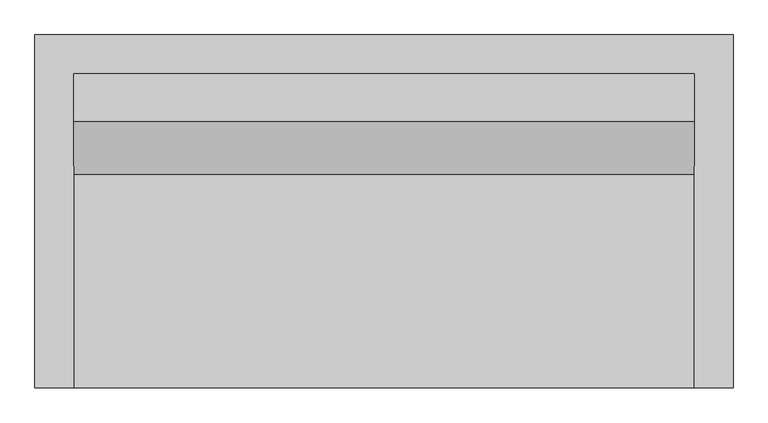
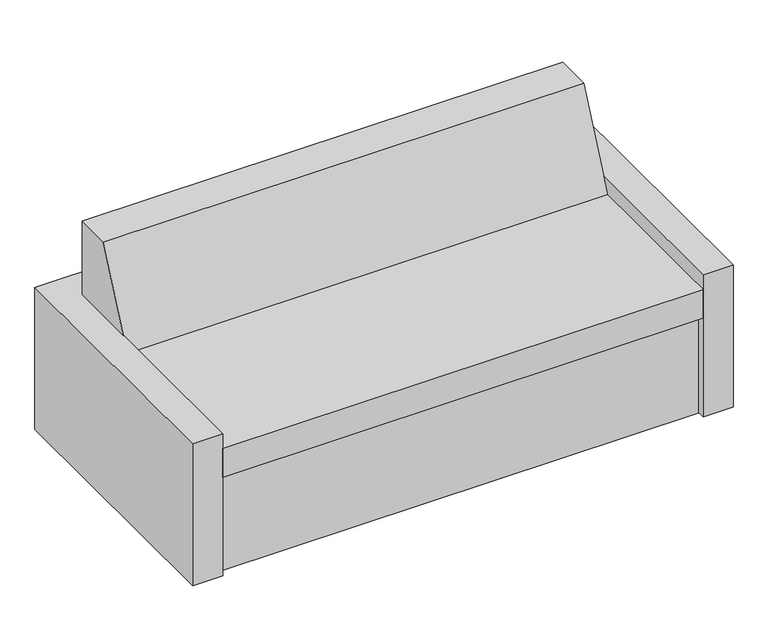
"""IFC4 building model written with IfcOpenShell, lengths in millimetres: furniture geometry."""

from ifc_helpers import new_model, si_unit, frame, origin, origin_with_axes, place, context, project, spatial, polyline, outline, extrude, source, transform, mapped, element, save


def furniture_703849cf(model_context):
    return source(origin(), model_context, "Body", "SweptSolid", [
        extrude(outline(polyline([(-359.4256442, 450.0), (-222.4208629, 760.0), (-100.0, 760.0), (-100.0, 0.0), (-884.6, 0.0), (-884.6, 348.4), (-910.0, 348.4), (-910.0, 450.0), (-359.4256442, 450.0)])), frame((-723.8, 0.0, 0.0), z_axis=(1.0, 0.0, 0.0), x_axis=(0.0, 1.0, 0.0)), (0.0, 0.0, 1.0), 1600.0),
        extrude(outline(polyline([(976.2, 0.0), (976.2, -910.0), (876.2, -910.0), (876.2, -100.0), (-723.8, -100.0), (-723.8, -910.0), (-823.8, -910.0), (-823.8, 0.0), (976.2, 0.0)])), origin_with_axes(), (0.0, 0.0, 1.0), 500.0),
    ])


if __name__ == "__main__":
    model = new_model("IFC4")
    model_context = context("Model", 3, world=origin())
    ifc_project = project(units=[si_unit("LENGTHUNIT", "METRE", prefix="MILLI")], contexts=[model_context])
    site = spatial("IfcSite", under=ifc_project)
    building = spatial("IfcBuilding", under=site)
    placement = place(None, origin())
    furniture_shape = furniture_703849cf(model_context)
    element("IfcFurniture", 1, at=placement, inside=building, context=model_context, shape_type="MappedRepresentation", body=[
        mapped(furniture_shape, transform((0.0, 0.0, 0.0), x_axis=(1.0, 0.0, 0.0), y_axis=(0.0, 1.0, 0.0), z_axis=(0.0, 0.0, 1.0))),
    ])
    save(model, "model.ifc")

# Revit data of these elements
# Type
#   width = 1800 mm
#   seat height = 450 mm
#   height = 760 mm
#   depth = 910 mm
#   arm height = 500 mm
#   arm depth = 100 mm
#   Total Seat Room = 1600 mm
#   Seat Width = 800 mm
#   Seat Count = 2
#   Is Mark Visible = yes
#   seat material = Sofa seat
#   arm material = Sofa arm
#   Default Elevation = 0
#   Assembly Code = ""
# Element 1 (IfcFurniture)
#   Materials on its faces: "Sofa seat", "Sofa arm"
# Materials
#   "Sofa seat": colour RGB 247 247 239, transparency 0
#   "Sofa arm": colour RGB 247 247 239, transparency 0
